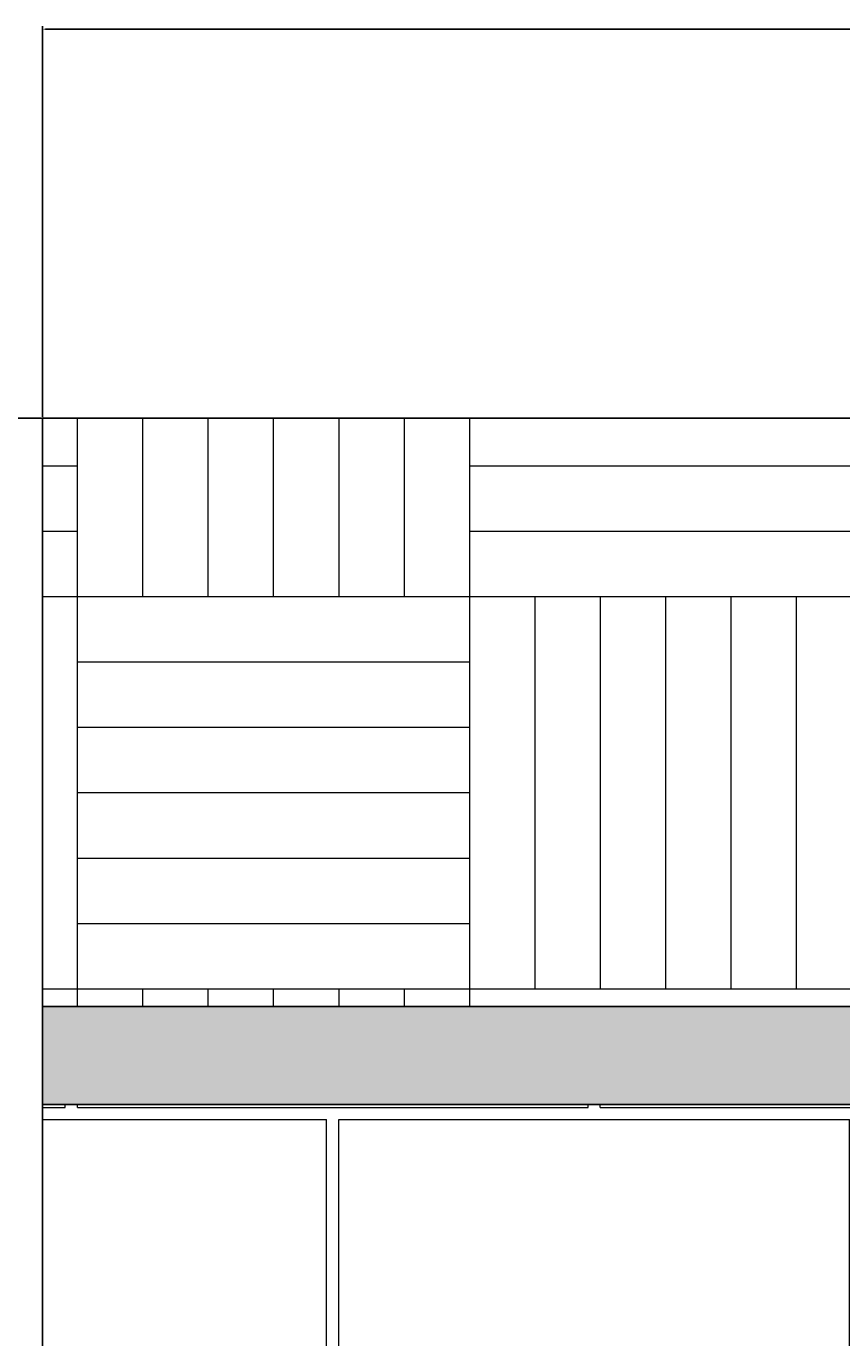
# Model space of a CAD drawing. Units: inches. Extents: x -128 to 854, y -395 to 398.
# Tile 58 of 61: x 417 to 467, y -248 to -167. Entities that reach past the tile are written whole.
import ezdxf

# ---------------------------------------------------------------- set-up
doc = ezdxf.new("R2010")
doc.units = ezdxf.units.IN
doc.header["$MEASUREMENT"] = 0
for name, color, linetype, lineweight in [('A-ANNO-DIMS', 2, 'Continuous', 18), ('A-ELEV', 3, 'Continuous', 25), ('A-ELEV-PATT', 8, 'Continuous', 13)]:
    doc.layers.add(name, color=color, linetype=linetype, lineweight=lineweight)
doc.styles.get("Standard").update_dxf_attribs({"font": 'arial.ttf'})
doc.dimstyles.get("Standard").update_dxf_attribs({"dimtxt": 0.18, "dimasz": 0.18, "dimexe": 0.18, "dimexo": 0.0625, "dimgap": 0.09, "dimtad": 0, "dimtih": 1, "dimtoh": 1, "dimdec": 1, "dimzin": 0, "dimdsep": 46, "dimlunit": 4, "dimtxsty": 'Standard', "dimcen": 0.09, "dimclrd": 1, "dimclre": 2, "dimclrt": 6, "dimadec": 0, "dimazin": 0, "dimtfac": 1, "dimtdec": 1, "dimtofl": 0, "dimtmove": 0, "dimatfit": 3, "dimfxl": 1, "dimtfill": 2, "dimtfillclr": 3, "dimtolj": 1, "dimtzin": 0, "dimarcsym": 0})

# ---------------------------------------------------------------- blocks, each defined once
blk = doc.blocks.new('*D133')
at = {"layer": 'A-ANNO-DIMS', "color": 2, "lineweight": -2, "transparency": 16777216}
for p, q in [((418.28, -191.414), (418.28, -167.496)), ((782.28, -191.414), (782.28, -167.496))]:
    blk.add_line(p, q, dxfattribs=at)
at = {"layer": 'A-ANNO-DIMS', "color": 1, "lineweight": -2, "transparency": 16777216}
for p, q in [((418.46, -167.676), (599.88, -167.676)), ((782.1, -167.676), (600.679, -167.676))]:
    blk.add_line(p, q, dxfattribs=at)
at = {"layer": 'A-ANNO-DIMS', "color": 1, "transparency": 16777216}
for points in [[(418.46, -167.646), (418.46, -167.706), (418.28, -167.676)], [(782.1, -167.646), (782.1, -167.706), (782.28, -167.676)]]:
    blk.add_solid(points, dxfattribs=at)
at = {"layer": 'Defpoints', "color": 0, "transparency": 16777216}
for p in [(782.28, -167.676), (418.28, -191.476), (782.28, -191.476)]:
    blk.add_point(p, dxfattribs=at)
at = {"layer": 'A-ANNO-DIMS', "color": 6, "transparency": 16777216, "insert": (600.28, -167.676), "char_height": 0.18, "attachment_point": 5, "bg_fill": 1, "box_fill_scale": 1.25, "bg_fill_color": 3, "bg_fill_transparency": 0}
blk.add_mtext('\\A1;30\'-4"', dxfattribs=at)
blk = doc.blocks.new('*D134')
at = {"layer": 'A-ANNO-DIMS', "color": 2, "lineweight": -2, "transparency": 16777216}
for p, q in [((418.217, -191.476), (346.3, -191.476)), ((418.217, -371.476), (346.3, -371.476))]:
    blk.add_line(p, q, dxfattribs=at)
at = {"layer": 'A-ANNO-DIMS', "color": 1, "lineweight": -2, "transparency": 16777216}
for p, q in [((346.48, -191.656), (346.48, -281.295)), ((346.48, -371.296), (346.48, -281.658))]:
    blk.add_line(p, q, dxfattribs=at)
at = {"layer": 'A-ANNO-DIMS', "color": 1, "transparency": 16777216}
for points in [[(346.45, -191.656), (346.51, -191.656), (346.48, -191.476)], [(346.45, -371.296), (346.51, -371.296), (346.48, -371.476)]]:
    blk.add_solid(points, dxfattribs=at)
at = {"layer": 'Defpoints', "color": 0, "transparency": 16777216}
for p in [(346.48, -191.476), (418.28, -191.476), (418.28, -371.476)]:
    blk.add_point(p, dxfattribs=at)
at = {"layer": 'A-ANNO-DIMS', "color": 6, "transparency": 16777216, "insert": (346.48, -281.476), "char_height": 0.18, "attachment_point": 5, "bg_fill": 1, "box_fill_scale": 1.25, "bg_fill_color": 3, "bg_fill_transparency": 0}
blk.add_mtext('\\A1;15\'-0"', dxfattribs=at)

msp = doc.modelspace()

# ---------------------------------------------------------------- hatches: boundary and pattern name
at = {"layer": 'A-ELEV-PATT'}
h = msp.add_hatch(dxfattribs=at)
h.set_pattern_fill('AR-PARQ1', color=256, scale=2)
h.set_pattern_definition([(90, (468.407, -10.41), (-24, 24), [24, -24]), (90, (472.407, -10.41), (-24, 24), [24, -24]), (90, (476.407, -10.41), (-24, 24), [24, -24]), (90, (480.407, -10.41), (-24, 24), [24, -24]), (90, (484.407, -10.41), (-24, 24), [24, -24]), (90, (488.407, -10.41), (-24, 24), [24, -24]), (90, (492.407, -10.41), (-24, 24), [24, -24]), (0, (468.407, 13.59), (24, -24), [24, -24]), (0, (468.407, 17.59), (24, -24), [24, -24]), (0, (468.407, 21.59), (24, -24), [24, -24]), (0, (468.407, 25.59), (24, -24), [24, -24]), (0, (468.407, 29.59), (24, -24), [24, -24]), (0, (468.407, 33.59), (24, -24), [24, -24]), (0, (468.407, 37.59), (24, -24), [24, -24])])
h.paths.add_polyline_path([(782.28, -227.476), (782.28, -191.476), (418.28, -191.476), (418.28, -227.476)])
h = msp.add_hatch(color=256, dxfattribs=at)
h.dxf.hatch_style = 1
h.paths.add_polyline_path([(418.28, -227.476), (418.28, -233.476), (782.28, -233.476), (782.28, -227.476)])
h.paths.add_polyline_path([(492.252, -257.476), (492.252, -353.476), (551.307, -353.476), (551.307, -257.476)])
h.paths.add_polyline_path([(546.307, -262.476), (546.307, -348.476), (497.252, -348.476), (497.252, -262.476)], flags=16)
h = msp.add_hatch(dxfattribs=at)
h.set_pattern_fill('AR-B816C', color=256, scale=2)
h.set_pattern_definition([(0, (468.407, -10.41), (16, 16), [31.25, -0.75]), (0, (452.407, -9.66), (16, 16), [31.25, -0.75]), (90, (468.407, -10.41), (-16, 16), [-16.75, 15.25]), (90, (467.657, -10.41), (-16, 16), [-16.75, 15.25])])
h.paths.add_polyline_path([(418.28, -353.476), (492.252, -353.476), (492.252, -257.476), (551.307, -257.476), (551.307, -353.476), (782.28, -353.476), (782.28, -233.476), (418.28, -233.476)])
h.paths.add_polyline_path([(668.28, -257.476), (730.28, -257.476), (730.28, -305.476), (668.28, -305.476)], flags=16)
h.paths.add_polyline_path([(673.28, -300.476), (673.28, -262.476), (725.28, -262.476), (725.28, -300.476)], flags=0)

# ---------------------------------------------------------------- linework, layer by layer
at = {"layer": 'A-ELEV'}
for points in [[(418.28, -191.476), (782.28, -191.476), (782.28, -227.476), (418.28, -227.476)], [(418.28, -227.476), (782.28, -227.476), (782.28, -233.476), (418.28, -233.476)], [(418.28, -233.476), (782.28, -233.476), (782.28, -353.476), (418.28, -353.476)]]:
    msp.add_lwpolyline(points, close=True, dxfattribs=at)

# ---------------------------------------------------------------- dimensions: what is measured, and where the dimension line sits
at = {"layer": 'A-ANNO-DIMS'}
dim = msp.add_linear_dim(base=(782.28, -167.676), p1=(418.28, -191.476), p2=(782.28, -191.476), dimstyle='Standard', override={"dimdec": 1, "dimlfac": 1, "dimrnd": 0, "dimzin": 1, "dimdsep": 46, "dimlunit": 4, "dimfrac": 2}, dxfattribs=at)
dim.commit()
dim.dimension.update_dxf_attribs({"geometry": '*D133', "text_midpoint": (600.28, -167.676)})
dim = msp.add_linear_dim(base=(346.48, -191.476), p1=(418.28, -371.476), p2=(418.28, -191.476), angle=90, dimstyle='Standard', override={"dimdec": 1, "dimlfac": 1, "dimrnd": 0, "dimzin": 1, "dimdsep": 46, "dimlunit": 4, "dimfrac": 2}, dxfattribs=at)
dim.commit()
dim.dimension.update_dxf_attribs({"geometry": '*D134', "text_midpoint": (346.48, -281.476)})

doc.saveas('drawing.dxf')
